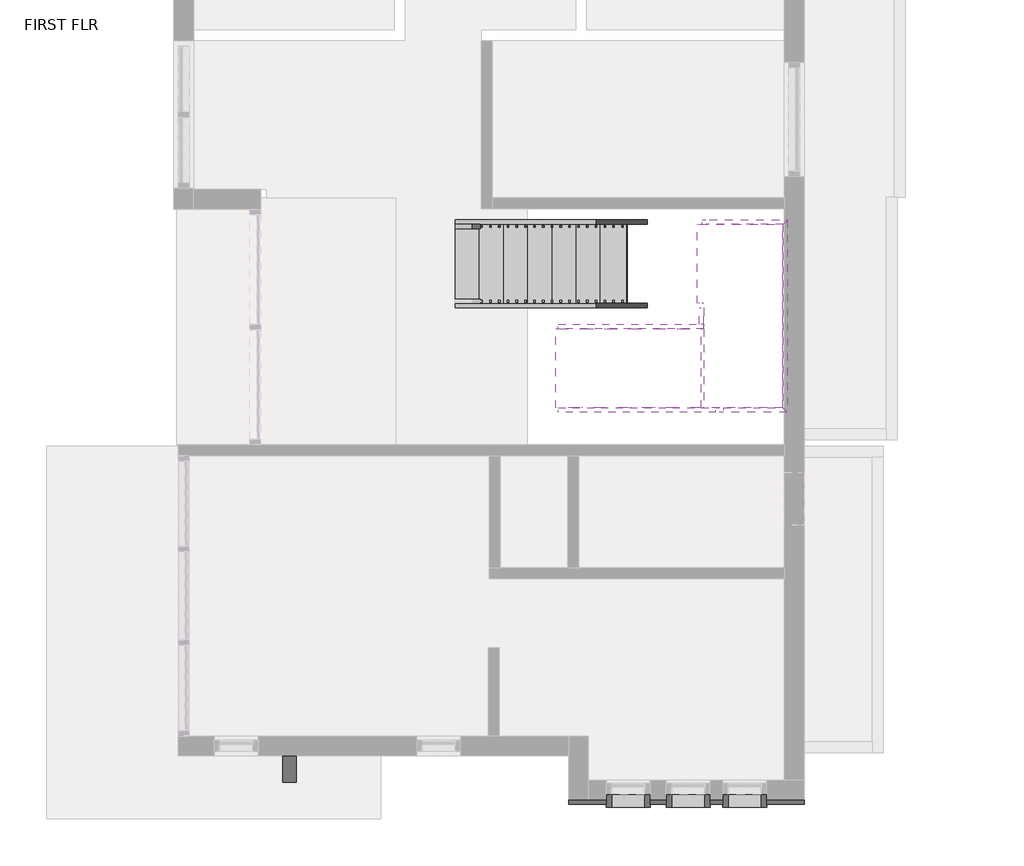
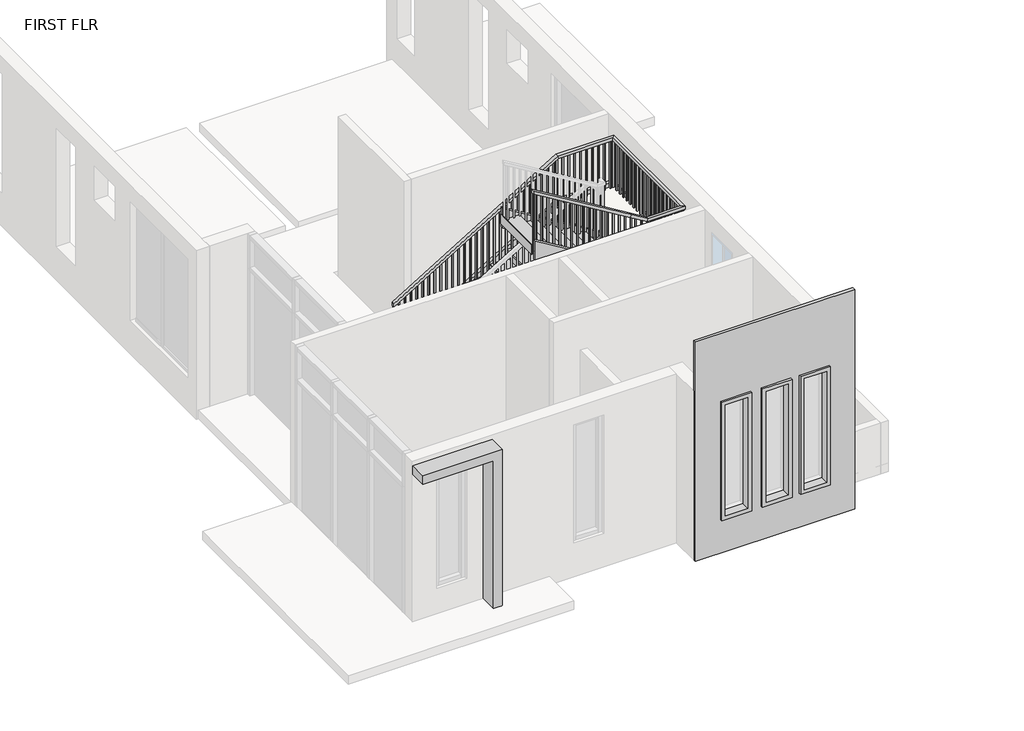
# One storey, part 4 of 4: 8 members, 3 proxies, 2 stair flights, 1 railing, 1 slab.
"""IFC4 building model written with IfcOpenShell, lengths in millimetres."""

from ifc_helpers import new_model, si_unit, frame, origin, place, context, project, spatial, polyline, outline, extrude, faceted_brep, transform, mapped, element, save
from components import generic_models_2_generic_models_2_65ba8ebd, generic_models_3_generic_models_3_7aa97fcf, generic_models_5_generic_models_5_32b8a8a5, non_monolithic_landing_a5fdca2b, stair_flight_bde5577f, stair_flight_bf40378d

model = new_model("IFC4")

# Units and contexts
model_context = context("Model", 3, world=origin())
ifc_project = project(units=[si_unit("LENGTHUNIT", "METRE", prefix="MILLI")], contexts=[model_context])

# Site, building, storey
site = spatial("IfcSite", under=ifc_project)
building = spatial("IfcBuilding", under=site)
storey = spatial("IfcBuildingStorey", under=building, Name="FIRST FLR", Elevation=3048.0)

# Proxies
placement = place(None, origin())
generic_models_2_generic_models_2_shape = generic_models_2_generic_models_2_65ba8ebd(model_context)
element("IfcBuildingElementProxy", 1, Name="Generic Models 2 : Generic Models 2", ObjectType="Generic Models 2 : Generic Models 2", at=placement, inside=storey, context=model_context, shape_type="MappedRepresentation", body=[
    mapped(generic_models_2_generic_models_2_shape, transform((0.0, 0.0, 0.0), x_axis=(1.0, 0.0, 0.0), y_axis=(0.0, 1.0, 0.0), z_axis=(0.0, 0.0, 1.0))),
])
generic_models_3_generic_models_3_shape = generic_models_3_generic_models_3_7aa97fcf(model_context)
element("IfcBuildingElementProxy", 2, Name="Generic Models 3 : Generic Models 3", ObjectType="Generic Models 3 : Generic Models 3", at=placement, inside=storey, context=model_context, shape_type="MappedRepresentation", body=[
    mapped(generic_models_3_generic_models_3_shape, transform((0.0, 0.0, 0.0), x_axis=(1.0, 0.0, 0.0), y_axis=(0.0, 1.0, 0.0), z_axis=(0.0, 0.0, 1.0))),
])
generic_models_5_generic_models_5_shape = generic_models_5_generic_models_5_32b8a8a5(model_context)
element("IfcBuildingElementProxy", 3, Name="Generic Models 5 : Generic Models 5", ObjectType="Generic Models 5 : Generic Models 5", at=placement, inside=storey, context=model_context, shape_type="MappedRepresentation", body=[
    mapped(generic_models_5_generic_models_5_shape, transform((0.0, 0.0, 0.0), x_axis=(1.0, 0.0, 0.0), y_axis=(0.0, 1.0, 0.0), z_axis=(0.0, 0.0, 1.0))),
])

# Members
element("IfcMember", 4, ObjectType="Stringer - 2\" Width", at=placement, inside=storey, context=model_context, shape_type="SweptSolid", body=[
    extrude(outline(polyline([(3260.114512, -9709.3703437), (3048.0, -9709.3703437), (3048.0, -9471.284832), (4682.0666667, -6775.074832), (4986.8666667, -6860.2292885), (3260.114512, -9709.3703437)])), frame((0.0, -5433.3504041, 0.0), z_axis=(0.0, 1.0, 0.0), x_axis=(0.0, 0.0, 1.0)), (0.0, 0.0, 1.0), 50.8),
])
element("IfcMember", 5, ObjectType="Stringer - 2\" Width", at=placement, inside=storey, context=model_context, shape_type="SweptSolid", body=[
    extrude(outline(polyline([(3260.114512, -9709.3703437), (3048.0, -9709.3703437), (3048.0, -9471.284832), (4641.9144067, -6841.3260609), (4986.8666667, -6841.3260609), (4986.8666667, -6860.2292885), (3260.114512, -9709.3703437)])), frame((0.0, -6398.5504041, 0.0), z_axis=(0.0, 1.0, 0.0), x_axis=(0.0, 0.0, 1.0)), (0.0, 0.0, 1.0), 50.8),
])
element("IfcMember", 6, ObjectType="Stringer - 2\" Width", at=placement, inside=storey, context=model_context, shape_type="SweptSolid", body=[
    extrude(outline(polyline([(4682.0666667, -6702.2215727), (4986.8666667, -6617.0671162), (6138.7811786, -8517.7260609), (5782.3724171, -8517.7260609), (4682.0666667, -6702.2215727)])), frame((0.0, -7604.2810793, 0.0), z_axis=(0.0, 1.0, 0.0), x_axis=(0.0, 0.0, 1.0)), (0.0, 0.0, 1.0), 50.8),
])
element("IfcMember", 7, ObjectType="Stringer - 2\" Width", at=placement, inside=storey, context=model_context, shape_type="SweptSolid", body=[
    extrude(outline(polyline([(4766.3724171, -6841.3260609), (5122.7811786, -6841.3260609), (6138.7811786, -8517.7260609), (5782.3724171, -8517.7260609), (4766.3724171, -6841.3260609)])), frame((0.0, -6639.0810793, 0.0), z_axis=(0.0, 1.0, 0.0), x_axis=(0.0, 0.0, 1.0)), (0.0, 0.0, 1.0), 50.8),
])
element("IfcMember", 8, ObjectType="Stringer - 2\" Width", at=placement, inside=storey, context=model_context, shape_type="Brep", body=[
    faceted_brep([(-6617.0671162, -7553.4810793, 4986.8666667), (-6617.0671162, -7604.2810793, 4986.8666667), (-5876.1260609, -7604.2810793, 4986.8666667), (-5926.9260609, -7553.4810793, 4986.8666667), (-6702.2215727, -7553.4810793, 4682.0666667), (-5926.9260609, -7553.4810793, 4682.0666667), (-6702.2215727, -7604.2810793, 4682.0666667), (-5876.1260609, -7604.2810793, 4682.0666667)], [[[0, 1, 2, 3]], [[4, 0, 3, 5]], [[6, 4, 5, 7]], [[1, 6, 7, 2]], [[1, 0, 4, 6]], [[2, 7, 5, 3]]]),
])
element("IfcMember", 9, ObjectType="Stringer - 2\" Width", at=placement, inside=storey, context=model_context, shape_type="SweptSolid", body=[
    extrude(outline(polyline([(-5876.1260609, -7604.2810793), (-5926.9260609, -7553.4810793), (-5926.9260609, -5433.3504041), (-5876.1260609, -5382.5504041), (-5876.1260609, -7604.2810793)])), frame((0.0, 0.0, 4682.0666667), z_axis=(0.0, 0.0, 1.0), x_axis=(1.0, 0.0, 0.0)), (0.0, 0.0, 1.0), 304.8),
])
element("IfcMember", 10, ObjectType="Stringer - 2\" Width", at=placement, inside=storey, context=model_context, shape_type="Brep", body=[
    faceted_brep([(-5926.9260609, -5433.3504041, 4986.8666667), (-5876.1260609, -5382.5504041, 4986.8666667), (-6860.2292885, -5382.5504041, 4986.8666667), (-6860.2292885, -5433.3504041, 4986.8666667), (-5926.9260609, -5433.3504041, 4682.0666667), (-6775.074832, -5433.3504041, 4682.0666667), (-5876.1260609, -5382.5504041, 4682.0666667), (-6775.074832, -5382.5504041, 4682.0666667)], [[[0, 1, 2, 3]], [[4, 0, 3, 5]], [[6, 4, 5, 7]], [[1, 6, 7, 2]], [[1, 0, 4, 6]], [[2, 7, 5, 3]]]),
])
element("IfcMember", 11, ObjectType="Stringer - 2\" Width", at=placement, inside=storey, context=model_context, shape_type="SweptSolid", body=[
    extrude(outline(polyline([(-6892.1260609, -6398.5504041), (-6841.3260609, -6398.5504041), (-6841.3260609, -6588.2810793), (-6892.1260609, -6588.2810793), (-6892.1260609, -6398.5504041)])), frame((0.0, 0.0, 4682.0666667), z_axis=(0.0, 0.0, 1.0), x_axis=(1.0, 0.0, 0.0)), (0.0, 0.0, 1.0), 304.8),
])

# Railing
element("IfcRailing", 12, ObjectType="Handrail - Rectangular", at=placement, inside=storey, context=model_context, shape_type="SolidModel", body=[
    faceted_brep([(-9709.3703437, -5433.3504041, 4131.7333333), (-9709.3703437, -5433.3504041, 4072.3318731), (-9709.3703437, -5484.1504041, 4072.3318731), (-9709.3703437, -5484.1504041, 4131.7333333), (-6915.3703437, -5433.3504041, 5825.0666667), (-6901.1779343, -5433.3504041, 5774.2666667), (-6901.1779343, -5484.1504041, 5774.2666667), (-6915.3703437, -5484.1504041, 5825.0666667), (-5926.9260609, -5433.3504041, 5825.0666667), (-5926.9260609, -5433.3504041, 5774.2666667), (-5977.7260609, -5484.1504041, 5774.2666667), (-5977.7260609, -5484.1504041, 5825.0666667), (-5926.9260609, -7553.4810793, 5825.0666667), (-5926.9260609, -7553.4810793, 5774.2666667), (-5977.7260609, -7502.6810793, 5774.2666667), (-5977.7260609, -7502.6810793, 5825.0666667), (-6561.9260609, -7553.4810793, 5825.0666667), (-6576.1184703, -7553.4810793, 5774.2666667), (-6576.1184703, -7502.6810793, 5774.2666667), (-6561.9260609, -7502.6810793, 5825.0666667), (-6841.3260609, -7553.4810793, 5994.4), (-6867.6557881, -7553.4810793, 5950.9559502), (-6867.6557881, -7502.6810793, 5950.9559502), (-6841.3260609, -7502.6810793, 5994.4), (-8517.7260609, -7553.4810793, 7010.4), (-8517.7260609, -7502.6810793, 7010.4), (-8517.7260609, -7502.6810793, 6950.9985397), (-8517.7260609, -7553.4810793, 6950.9985397)], [[[0, 1, 2, 3]], [[1, 0, 4, 5]], [[2, 1, 5, 6]], [[3, 2, 6, 7]], [[0, 3, 7, 4]], [[5, 4, 8, 9]], [[6, 5, 9, 10]], [[7, 6, 10, 11]], [[4, 7, 11, 8]], [[9, 8, 12, 13]], [[10, 9, 13, 14]], [[11, 10, 14, 15]], [[8, 11, 15, 12]], [[13, 12, 16, 17]], [[14, 13, 17, 18]], [[15, 14, 18, 19]], [[12, 15, 19, 16]], [[17, 16, 20, 21]], [[18, 17, 21, 22]], [[19, 18, 22, 23]], [[16, 19, 23, 20]], [[24, 25, 26, 27]], [[21, 20, 24, 27]], [[22, 21, 27, 26]], [[23, 22, 26, 25]], [[20, 23, 25, 24]]]),
    extrude(outline(polyline([(6925.9833882, -8476.4510609), (5926.6666667, -8476.4510609), (5926.6666667, -8457.4010609), (6914.4379337, -8457.4010609), (6925.9833882, -8476.4510609)])), frame((0.0, -7537.6060793, 0.0), z_axis=(0.0, 1.0, 0.0), x_axis=(0.0, 0.0, 1.0)), (0.0, 0.0, 1.0), 19.05),
    extrude(outline(polyline([(6864.4076307, -8374.8510609), (5926.6666667, -8374.8510609), (5926.6666667, -8355.8010609), (6852.8621761, -8355.8010609), (6864.4076307, -8374.8510609)])), frame((0.0, -7537.6060793, 0.0), z_axis=(0.0, 1.0, 0.0), x_axis=(0.0, 0.0, 1.0)), (0.0, 0.0, 1.0), 19.05),
    extrude(outline(polyline([(6802.8318731, -8273.2510609), (5926.6666667, -8273.2510609), (5926.6666667, -8254.2010609), (6791.2864185, -8254.2010609), (6802.8318731, -8273.2510609)])), frame((0.0, -7537.6060793, 0.0), z_axis=(0.0, 1.0, 0.0), x_axis=(0.0, 0.0, 1.0)), (0.0, 0.0, 1.0), 19.05),
    extrude(outline(polyline([(6741.2561155, -8171.6510609), (5757.3333333, -8171.6510609), (5757.3333333, -8152.6010609), (6729.710661, -8152.6010609), (6741.2561155, -8171.6510609)])), frame((0.0, -7537.6060793, 0.0), z_axis=(0.0, 1.0, 0.0), x_axis=(0.0, 0.0, 1.0)), (0.0, 0.0, 1.0), 19.05),
    extrude(outline(polyline([(6679.6803579, -8070.0510609), (5757.3333333, -8070.0510609), (5757.3333333, -8051.0010609), (6668.1349034, -8051.0010609), (6679.6803579, -8070.0510609)])), frame((0.0, -7537.6060793, 0.0), z_axis=(0.0, 1.0, 0.0), x_axis=(0.0, 0.0, 1.0)), (0.0, 0.0, 1.0), 19.05),
    extrude(outline(polyline([(6618.1046004, -7968.4510609), (5757.3333333, -7968.4510609), (5757.3333333, -7949.4010609), (6606.5591458, -7949.4010609), (6618.1046004, -7968.4510609)])), frame((0.0, -7537.6060793, 0.0), z_axis=(0.0, 1.0, 0.0), x_axis=(0.0, 0.0, 1.0)), (0.0, 0.0, 1.0), 19.05),
    extrude(outline(polyline([(6556.5288428, -7866.8510609), (5588.0, -7866.8510609), (5588.0, -7847.8010609), (6544.9833882, -7847.8010609), (6556.5288428, -7866.8510609)])), frame((0.0, -7537.6060793, 0.0), z_axis=(0.0, 1.0, 0.0), x_axis=(0.0, 0.0, 1.0)), (0.0, 0.0, 1.0), 19.05),
    extrude(outline(polyline([(6494.9530852, -7765.2510609), (5588.0, -7765.2510609), (5588.0, -7746.2010609), (6483.4076307, -7746.2010609), (6494.9530852, -7765.2510609)])), frame((0.0, -7537.6060793, 0.0), z_axis=(0.0, 1.0, 0.0), x_axis=(0.0, 0.0, 1.0)), (0.0, 0.0, 1.0), 19.05),
    extrude(outline(polyline([(6433.3773276, -7663.6510609), (5418.6666667, -7663.6510609), (5418.6666667, -7644.6010609), (6421.8318731, -7644.6010609), (6433.3773276, -7663.6510609)])), frame((0.0, -7537.6060793, 0.0), z_axis=(0.0, 1.0, 0.0), x_axis=(0.0, 0.0, 1.0)), (0.0, 0.0, 1.0), 19.05),
    extrude(outline(polyline([(6371.80157, -7562.0510609), (5418.6666667, -7562.0510609), (5418.6666667, -7543.0010609), (6360.2561155, -7543.0010609), (6371.80157, -7562.0510609)])), frame((0.0, -7537.6060793, 0.0), z_axis=(0.0, 1.0, 0.0), x_axis=(0.0, 0.0, 1.0)), (0.0, 0.0, 1.0), 19.05),
    extrude(outline(polyline([(6310.2258125, -7460.4510609), (5418.6666667, -7460.4510609), (5418.6666667, -7441.4010609), (6298.6803579, -7441.4010609), (6310.2258125, -7460.4510609)])), frame((0.0, -7537.6060793, 0.0), z_axis=(0.0, 1.0, 0.0), x_axis=(0.0, 0.0, 1.0)), (0.0, 0.0, 1.0), 19.05),
    extrude(outline(polyline([(6248.6500549, -7358.8510609), (5249.3333333, -7358.8510609), (5249.3333333, -7339.8010609), (6237.1046004, -7339.8010609), (6248.6500549, -7358.8510609)])), frame((0.0, -7537.6060793, 0.0), z_axis=(0.0, 1.0, 0.0), x_axis=(0.0, 0.0, 1.0)), (0.0, 0.0, 1.0), 19.05),
    extrude(outline(polyline([(6187.0742973, -7257.2510609), (5249.3333333, -7257.2510609), (5249.3333333, -7238.2010609), (6175.5288428, -7238.2010609), (6187.0742973, -7257.2510609)])), frame((0.0, -7537.6060793, 0.0), z_axis=(0.0, 1.0, 0.0), x_axis=(0.0, 0.0, 1.0)), (0.0, 0.0, 1.0), 19.05),
    extrude(outline(polyline([(6125.4985397, -7155.6510609), (5249.3333333, -7155.6510609), (5249.3333333, -7136.6010609), (6113.9530852, -7136.6010609), (6125.4985397, -7155.6510609)])), frame((0.0, -7537.6060793, 0.0), z_axis=(0.0, 1.0, 0.0), x_axis=(0.0, 0.0, 1.0)), (0.0, 0.0, 1.0), 19.05),
    extrude(outline(polyline([(6063.9227822, -7054.0510609), (5080.0, -7054.0510609), (5080.0, -7035.0010609), (6052.3773276, -7035.0010609), (6063.9227822, -7054.0510609)])), frame((0.0, -7537.6060793, 0.0), z_axis=(0.0, 1.0, 0.0), x_axis=(0.0, 0.0, 1.0)), (0.0, 0.0, 1.0), 19.05),
    extrude(outline(polyline([(6002.3470246, -6952.4510609), (5080.0, -6952.4510609), (5080.0, -6933.4010609), (5990.80157, -6933.4010609), (6002.3470246, -6952.4510609)])), frame((0.0, -7537.6060793, 0.0), z_axis=(0.0, 1.0, 0.0), x_axis=(0.0, 0.0, 1.0)), (0.0, 0.0, 1.0), 19.05),
    extrude(outline(polyline([(5894.5894488, -6774.6510609), (4910.6666667, -6774.6510609), (4910.6666667, -6755.6010609), (5883.0439943, -6755.6010609), (5894.5894488, -6774.6510609)])), frame((0.0, -7537.6060793, 0.0), z_axis=(0.0, 1.0, 0.0), x_axis=(0.0, 0.0, 1.0)), (0.0, 0.0, 1.0), 19.05),
    extrude(outline(polyline([(5833.0136913, -6673.0510609), (4910.6666667, -6673.0510609), (4910.6666667, -6654.0010609), (5821.4682367, -6654.0010609), (5833.0136913, -6673.0510609)])), frame((0.0, -7537.6060793, 0.0), z_axis=(0.0, 1.0, 0.0), x_axis=(0.0, 0.0, 1.0)), (0.0, 0.0, 1.0), 19.05),
    extrude(outline(polyline([(-6552.4010609, -7537.6060793), (-6571.4510609, -7537.6060793), (-6571.4510609, -7518.5560793), (-6552.4010609, -7518.5560793), (-6552.4010609, -7537.6060793)])), frame((0.0, 0.0, 4910.6666667), z_axis=(0.0, 0.0, 1.0), x_axis=(1.0, 0.0, 0.0)), (0.0, 0.0, 1.0), 863.6),
    extrude(outline(polyline([(-6450.8010609, -7537.6060793), (-6469.8510609, -7537.6060793), (-6469.8510609, -7518.5560793), (-6450.8010609, -7518.5560793), (-6450.8010609, -7537.6060793)])), frame((0.0, 0.0, 4910.6666667), z_axis=(0.0, 0.0, 1.0), x_axis=(1.0, 0.0, 0.0)), (0.0, 0.0, 1.0), 863.6),
    extrude(outline(polyline([(-6349.2010609, -7537.6060793), (-6368.2510609, -7537.6060793), (-6368.2510609, -7518.5560793), (-6349.2010609, -7518.5560793), (-6349.2010609, -7537.6060793)])), frame((0.0, 0.0, 4910.6666667), z_axis=(0.0, 0.0, 1.0), x_axis=(1.0, 0.0, 0.0)), (0.0, 0.0, 1.0), 863.6),
    extrude(outline(polyline([(-6247.6010609, -7537.6060793), (-6266.6510609, -7537.6060793), (-6266.6510609, -7518.5560793), (-6247.6010609, -7518.5560793), (-6247.6010609, -7537.6060793)])), frame((0.0, 0.0, 4910.6666667), z_axis=(0.0, 0.0, 1.0), x_axis=(1.0, 0.0, 0.0)), (0.0, 0.0, 1.0), 863.6),
    extrude(outline(polyline([(-6146.0010609, -7537.6060793), (-6165.0510609, -7537.6060793), (-6165.0510609, -7518.5560793), (-6146.0010609, -7518.5560793), (-6146.0010609, -7537.6060793)])), frame((0.0, 0.0, 4910.6666667), z_axis=(0.0, 0.0, 1.0), x_axis=(1.0, 0.0, 0.0)), (0.0, 0.0, 1.0), 863.6),
    extrude(outline(polyline([(-6044.4010609, -7537.6060793), (-6063.4510609, -7537.6060793), (-6063.4510609, -7518.5560793), (-6044.4010609, -7518.5560793), (-6044.4010609, -7537.6060793)])), frame((0.0, 0.0, 4910.6666667), z_axis=(0.0, 0.0, 1.0), x_axis=(1.0, 0.0, 0.0)), (0.0, 0.0, 1.0), 863.6),
    extrude(outline(polyline([(-5942.8010609, -7481.2254041), (-5942.8010609, -7500.2754041), (-5961.8510609, -7500.2754041), (-5961.8510609, -7481.2254041), (-5942.8010609, -7481.2254041)])), frame((0.0, 0.0, 4910.6666667), z_axis=(0.0, 0.0, 1.0), x_axis=(1.0, 0.0, 0.0)), (0.0, 0.0, 1.0), 863.6),
    extrude(outline(polyline([(-5942.8010609, -7379.6254041), (-5942.8010609, -7398.6754041), (-5961.8510609, -7398.6754041), (-5961.8510609, -7379.6254041), (-5942.8010609, -7379.6254041)])), frame((0.0, 0.0, 4910.6666667), z_axis=(0.0, 0.0, 1.0), x_axis=(1.0, 0.0, 0.0)), (0.0, 0.0, 1.0), 863.6),
    extrude(outline(polyline([(-5942.8010609, -7278.0254041), (-5942.8010609, -7297.0754041), (-5961.8510609, -7297.0754041), (-5961.8510609, -7278.0254041), (-5942.8010609, -7278.0254041)])), frame((0.0, 0.0, 4910.6666667), z_axis=(0.0, 0.0, 1.0), x_axis=(1.0, 0.0, 0.0)), (0.0, 0.0, 1.0), 863.6),
    extrude(outline(polyline([(-5942.8010609, -7176.4254041), (-5942.8010609, -7195.4754041), (-5961.8510609, -7195.4754041), (-5961.8510609, -7176.4254041), (-5942.8010609, -7176.4254041)])), frame((0.0, 0.0, 4910.6666667), z_axis=(0.0, 0.0, 1.0), x_axis=(1.0, 0.0, 0.0)), (0.0, 0.0, 1.0), 863.6),
    extrude(outline(polyline([(-5942.8010609, -7074.8254041), (-5942.8010609, -7093.8754041), (-5961.8510609, -7093.8754041), (-5961.8510609, -7074.8254041), (-5942.8010609, -7074.8254041)])), frame((0.0, 0.0, 4910.6666667), z_axis=(0.0, 0.0, 1.0), x_axis=(1.0, 0.0, 0.0)), (0.0, 0.0, 1.0), 863.6),
    extrude(outline(polyline([(-5942.8010609, -6973.2254041), (-5942.8010609, -6992.2754041), (-5961.8510609, -6992.2754041), (-5961.8510609, -6973.2254041), (-5942.8010609, -6973.2254041)])), frame((0.0, 0.0, 4910.6666667), z_axis=(0.0, 0.0, 1.0), x_axis=(1.0, 0.0, 0.0)), (0.0, 0.0, 1.0), 863.6),
    extrude(outline(polyline([(-5942.8010609, -6871.6254041), (-5942.8010609, -6890.6754041), (-5961.8510609, -6890.6754041), (-5961.8510609, -6871.6254041), (-5942.8010609, -6871.6254041)])), frame((0.0, 0.0, 4910.6666667), z_axis=(0.0, 0.0, 1.0), x_axis=(1.0, 0.0, 0.0)), (0.0, 0.0, 1.0), 863.6),
    extrude(outline(polyline([(-5942.8010609, -6770.0254041), (-5942.8010609, -6789.0754041), (-5961.8510609, -6789.0754041), (-5961.8510609, -6770.0254041), (-5942.8010609, -6770.0254041)])), frame((0.0, 0.0, 4910.6666667), z_axis=(0.0, 0.0, 1.0), x_axis=(1.0, 0.0, 0.0)), (0.0, 0.0, 1.0), 863.6),
    extrude(outline(polyline([(-5942.8010609, -6668.4254041), (-5942.8010609, -6687.4754041), (-5961.8510609, -6687.4754041), (-5961.8510609, -6668.4254041), (-5942.8010609, -6668.4254041)])), frame((0.0, 0.0, 4910.6666667), z_axis=(0.0, 0.0, 1.0), x_axis=(1.0, 0.0, 0.0)), (0.0, 0.0, 1.0), 863.6),
    extrude(outline(polyline([(-5942.8010609, -6566.8254041), (-5942.8010609, -6585.8754041), (-5961.8510609, -6585.8754041), (-5961.8510609, -6566.8254041), (-5942.8010609, -6566.8254041)])), frame((0.0, 0.0, 4910.6666667), z_axis=(0.0, 0.0, 1.0), x_axis=(1.0, 0.0, 0.0)), (0.0, 0.0, 1.0), 863.6),
    extrude(outline(polyline([(-5942.8010609, -6465.2254041), (-5942.8010609, -6484.2754041), (-5961.8510609, -6484.2754041), (-5961.8510609, -6465.2254041), (-5942.8010609, -6465.2254041)])), frame((0.0, 0.0, 4910.6666667), z_axis=(0.0, 0.0, 1.0), x_axis=(1.0, 0.0, 0.0)), (0.0, 0.0, 1.0), 863.6),
    extrude(outline(polyline([(-5942.8010609, -6363.6254041), (-5942.8010609, -6382.6754041), (-5961.8510609, -6382.6754041), (-5961.8510609, -6363.6254041), (-5942.8010609, -6363.6254041)])), frame((0.0, 0.0, 4910.6666667), z_axis=(0.0, 0.0, 1.0), x_axis=(1.0, 0.0, 0.0)), (0.0, 0.0, 1.0), 863.6),
    extrude(outline(polyline([(-5942.8010609, -6262.0254041), (-5942.8010609, -6281.0754041), (-5961.8510609, -6281.0754041), (-5961.8510609, -6262.0254041), (-5942.8010609, -6262.0254041)])), frame((0.0, 0.0, 4910.6666667), z_axis=(0.0, 0.0, 1.0), x_axis=(1.0, 0.0, 0.0)), (0.0, 0.0, 1.0), 863.6),
    extrude(outline(polyline([(-5942.8010609, -6160.4254041), (-5942.8010609, -6179.4754041), (-5961.8510609, -6179.4754041), (-5961.8510609, -6160.4254041), (-5942.8010609, -6160.4254041)])), frame((0.0, 0.0, 4910.6666667), z_axis=(0.0, 0.0, 1.0), x_axis=(1.0, 0.0, 0.0)), (0.0, 0.0, 1.0), 863.6),
    extrude(outline(polyline([(-5942.8010609, -6058.8254041), (-5942.8010609, -6077.8754041), (-5961.8510609, -6077.8754041), (-5961.8510609, -6058.8254041), (-5942.8010609, -6058.8254041)])), frame((0.0, 0.0, 4910.6666667), z_axis=(0.0, 0.0, 1.0), x_axis=(1.0, 0.0, 0.0)), (0.0, 0.0, 1.0), 863.6),
    extrude(outline(polyline([(-5942.8010609, -5957.2254041), (-5942.8010609, -5976.2754041), (-5961.8510609, -5976.2754041), (-5961.8510609, -5957.2254041), (-5942.8010609, -5957.2254041)])), frame((0.0, 0.0, 4910.6666667), z_axis=(0.0, 0.0, 1.0), x_axis=(1.0, 0.0, 0.0)), (0.0, 0.0, 1.0), 863.6),
    extrude(outline(polyline([(-5942.8010609, -5855.6254041), (-5942.8010609, -5874.6754041), (-5961.8510609, -5874.6754041), (-5961.8510609, -5855.6254041), (-5942.8010609, -5855.6254041)])), frame((0.0, 0.0, 4910.6666667), z_axis=(0.0, 0.0, 1.0), x_axis=(1.0, 0.0, 0.0)), (0.0, 0.0, 1.0), 863.6),
    extrude(outline(polyline([(-5942.8010609, -5754.0254041), (-5942.8010609, -5773.0754041), (-5961.8510609, -5773.0754041), (-5961.8510609, -5754.0254041), (-5942.8010609, -5754.0254041)])), frame((0.0, 0.0, 4910.6666667), z_axis=(0.0, 0.0, 1.0), x_axis=(1.0, 0.0, 0.0)), (0.0, 0.0, 1.0), 863.6),
    extrude(outline(polyline([(-5942.8010609, -5652.4254041), (-5942.8010609, -5671.4754041), (-5961.8510609, -5671.4754041), (-5961.8510609, -5652.4254041), (-5942.8010609, -5652.4254041)])), frame((0.0, 0.0, 4910.6666667), z_axis=(0.0, 0.0, 1.0), x_axis=(1.0, 0.0, 0.0)), (0.0, 0.0, 1.0), 863.6),
    extrude(outline(polyline([(-5942.8010609, -5550.8254041), (-5942.8010609, -5569.8754041), (-5961.8510609, -5569.8754041), (-5961.8510609, -5550.8254041), (-5942.8010609, -5550.8254041)])), frame((0.0, 0.0, 4910.6666667), z_axis=(0.0, 0.0, 1.0), x_axis=(1.0, 0.0, 0.0)), (0.0, 0.0, 1.0), 863.6),
    extrude(outline(polyline([(-6010.4953437, -5449.2254041), (-5991.4453437, -5449.2254041), (-5991.4453437, -5468.2754041), (-6010.4953437, -5468.2754041), (-6010.4953437, -5449.2254041)])), frame((0.0, 0.0, 4910.6666667), z_axis=(0.0, 0.0, 1.0), x_axis=(1.0, 0.0, 0.0)), (0.0, 0.0, 1.0), 863.6),
    extrude(outline(polyline([(-6112.0953437, -5449.2254041), (-6093.0453437, -5449.2254041), (-6093.0453437, -5468.2754041), (-6112.0953437, -5468.2754041), (-6112.0953437, -5449.2254041)])), frame((0.0, 0.0, 4910.6666667), z_axis=(0.0, 0.0, 1.0), x_axis=(1.0, 0.0, 0.0)), (0.0, 0.0, 1.0), 863.6),
    extrude(outline(polyline([(-6213.6953437, -5449.2254041), (-6194.6453437, -5449.2254041), (-6194.6453437, -5468.2754041), (-6213.6953437, -5468.2754041), (-6213.6953437, -5449.2254041)])), frame((0.0, 0.0, 4910.6666667), z_axis=(0.0, 0.0, 1.0), x_axis=(1.0, 0.0, 0.0)), (0.0, 0.0, 1.0), 863.6),
    extrude(outline(polyline([(-6315.2953437, -5449.2254041), (-6296.2453437, -5449.2254041), (-6296.2453437, -5468.2754041), (-6315.2953437, -5468.2754041), (-6315.2953437, -5449.2254041)])), frame((0.0, 0.0, 4910.6666667), z_axis=(0.0, 0.0, 1.0), x_axis=(1.0, 0.0, 0.0)), (0.0, 0.0, 1.0), 863.6),
    extrude(outline(polyline([(-6416.8953437, -5449.2254041), (-6397.8453437, -5449.2254041), (-6397.8453437, -5468.2754041), (-6416.8953437, -5468.2754041), (-6416.8953437, -5449.2254041)])), frame((0.0, 0.0, 4910.6666667), z_axis=(0.0, 0.0, 1.0), x_axis=(1.0, 0.0, 0.0)), (0.0, 0.0, 1.0), 863.6),
    extrude(outline(polyline([(-6518.4953437, -5449.2254041), (-6499.4453437, -5449.2254041), (-6499.4453437, -5468.2754041), (-6518.4953437, -5468.2754041), (-6518.4953437, -5449.2254041)])), frame((0.0, 0.0, 4910.6666667), z_axis=(0.0, 0.0, 1.0), x_axis=(1.0, 0.0, 0.0)), (0.0, 0.0, 1.0), 863.6),
    extrude(outline(polyline([(-6620.0953437, -5449.2254041), (-6601.0453437, -5449.2254041), (-6601.0453437, -5468.2754041), (-6620.0953437, -5468.2754041), (-6620.0953437, -5449.2254041)])), frame((0.0, 0.0, 4910.6666667), z_axis=(0.0, 0.0, 1.0), x_axis=(1.0, 0.0, 0.0)), (0.0, 0.0, 1.0), 863.6),
    extrude(outline(polyline([(-6721.6953437, -5449.2254041), (-6702.6453437, -5449.2254041), (-6702.6453437, -5468.2754041), (-6721.6953437, -5468.2754041), (-6721.6953437, -5449.2254041)])), frame((0.0, 0.0, 4910.6666667), z_axis=(0.0, 0.0, 1.0), x_axis=(1.0, 0.0, 0.0)), (0.0, 0.0, 1.0), 863.6),
    extrude(outline(polyline([(-6823.2953437, -5449.2254041), (-6804.2453437, -5449.2254041), (-6804.2453437, -5468.2754041), (-6823.2953437, -5468.2754041), (-6823.2953437, -5449.2254041)])), frame((0.0, 0.0, 4910.6666667), z_axis=(0.0, 0.0, 1.0), x_axis=(1.0, 0.0, 0.0)), (0.0, 0.0, 1.0), 863.6),
    extrude(outline(polyline([(5729.1046004, -6975.6953437), (4741.3333333, -6975.6953437), (4741.3333333, -6956.6453437), (5740.6500549, -6956.6453437), (5729.1046004, -6975.6953437)])), frame((0.0, -5468.2754041, 0.0), z_axis=(0.0, 1.0, 0.0), x_axis=(0.0, 0.0, 1.0)), (0.0, 0.0, 1.0), 19.05),
    extrude(outline(polyline([(5667.5288428, -7077.2953437), (4741.3333333, -7077.2953437), (4741.3333333, -7058.2453437), (5679.0742973, -7058.2453437), (5667.5288428, -7077.2953437)])), frame((0.0, -5468.2754041, 0.0), z_axis=(0.0, 1.0, 0.0), x_axis=(0.0, 0.0, 1.0)), (0.0, 0.0, 1.0), 19.05),
    extrude(outline(polyline([(5605.9530852, -7178.8953437), (4741.3333333, -7178.8953437), (4741.3333333, -7159.8453437), (5617.4985397, -7159.8453437), (5605.9530852, -7178.8953437)])), frame((0.0, -5468.2754041, 0.0), z_axis=(0.0, 1.0, 0.0), x_axis=(0.0, 0.0, 1.0)), (0.0, 0.0, 1.0), 19.05),
    extrude(outline(polyline([(5544.3773276, -7280.4953437), (4572.0, -7280.4953437), (4572.0, -7261.4453437), (5555.9227822, -7261.4453437), (5544.3773276, -7280.4953437)])), frame((0.0, -5468.2754041, 0.0), z_axis=(0.0, 1.0, 0.0), x_axis=(0.0, 0.0, 1.0)), (0.0, 0.0, 1.0), 19.05),
    extrude(outline(polyline([(5482.80157, -7382.0953437), (4572.0, -7382.0953437), (4572.0, -7363.0453437), (5494.3470246, -7363.0453437), (5482.80157, -7382.0953437)])), frame((0.0, -5468.2754041, 0.0), z_axis=(0.0, 1.0, 0.0), x_axis=(0.0, 0.0, 1.0)), (0.0, 0.0, 1.0), 19.05),
    extrude(outline(polyline([(5421.2258125, -7483.6953437), (4572.0, -7483.6953437), (4572.0, -7464.6453437), (5432.771267, -7464.6453437), (5421.2258125, -7483.6953437)])), frame((0.0, -5468.2754041, 0.0), z_axis=(0.0, 1.0, 0.0), x_axis=(0.0, 0.0, 1.0)), (0.0, 0.0, 1.0), 19.05),
    extrude(outline(polyline([(5359.6500549, -7585.2953437), (4402.6666667, -7585.2953437), (4402.6666667, -7566.2453437), (5371.1955094, -7566.2453437), (5359.6500549, -7585.2953437)])), frame((0.0, -5468.2754041, 0.0), z_axis=(0.0, 1.0, 0.0), x_axis=(0.0, 0.0, 1.0)), (0.0, 0.0, 1.0), 19.05),
    extrude(outline(polyline([(5298.0742973, -7686.8953437), (4402.6666667, -7686.8953437), (4402.6666667, -7667.8453437), (5309.6197519, -7667.8453437), (5298.0742973, -7686.8953437)])), frame((0.0, -5468.2754041, 0.0), z_axis=(0.0, 1.0, 0.0), x_axis=(0.0, 0.0, 1.0)), (0.0, 0.0, 1.0), 19.05),
    extrude(outline(polyline([(5236.4985397, -7788.4953437), (4233.3333333, -7788.4953437), (4233.3333333, -7769.4453437), (5248.0439943, -7769.4453437), (5236.4985397, -7788.4953437)])), frame((0.0, -5468.2754041, 0.0), z_axis=(0.0, 1.0, 0.0), x_axis=(0.0, 0.0, 1.0)), (0.0, 0.0, 1.0), 19.05),
    extrude(outline(polyline([(5174.9227822, -7890.0953437), (4233.3333333, -7890.0953437), (4233.3333333, -7871.0453437), (5186.4682367, -7871.0453437), (5174.9227822, -7890.0953437)])), frame((0.0, -5468.2754041, 0.0), z_axis=(0.0, 1.0, 0.0), x_axis=(0.0, 0.0, 1.0)), (0.0, 0.0, 1.0), 19.05),
    extrude(outline(polyline([(5113.3470246, -7991.6953437), (4233.3333333, -7991.6953437), (4233.3333333, -7972.6453437), (5124.8924791, -7972.6453437), (5113.3470246, -7991.6953437)])), frame((0.0, -5468.2754041, 0.0), z_axis=(0.0, 1.0, 0.0), x_axis=(0.0, 0.0, 1.0)), (0.0, 0.0, 1.0), 19.05),
    extrude(outline(polyline([(5051.771267, -8093.2953437), (4064.0, -8093.2953437), (4064.0, -8074.2453437), (5063.3167216, -8074.2453437), (5051.771267, -8093.2953437)])), frame((0.0, -5468.2754041, 0.0), z_axis=(0.0, 1.0, 0.0), x_axis=(0.0, 0.0, 1.0)), (0.0, 0.0, 1.0), 19.05),
    extrude(outline(polyline([(4990.1955094, -8194.8953437), (4064.0, -8194.8953437), (4064.0, -8175.8453437), (5001.740964, -8175.8453437), (4990.1955094, -8194.8953437)])), frame((0.0, -5468.2754041, 0.0), z_axis=(0.0, 1.0, 0.0), x_axis=(0.0, 0.0, 1.0)), (0.0, 0.0, 1.0), 19.05),
    extrude(outline(polyline([(4928.6197519, -8296.4953437), (4064.0, -8296.4953437), (4064.0, -8277.4453437), (4940.1652064, -8277.4453437), (4928.6197519, -8296.4953437)])), frame((0.0, -5468.2754041, 0.0), z_axis=(0.0, 1.0, 0.0), x_axis=(0.0, 0.0, 1.0)), (0.0, 0.0, 1.0), 19.05),
    extrude(outline(polyline([(4867.0439943, -8398.0953437), (3894.6666667, -8398.0953437), (3894.6666667, -8379.0453437), (4878.5894488, -8379.0453437), (4867.0439943, -8398.0953437)])), frame((0.0, -5468.2754041, 0.0), z_axis=(0.0, 1.0, 0.0), x_axis=(0.0, 0.0, 1.0)), (0.0, 0.0, 1.0), 19.05),
    extrude(outline(polyline([(4805.4682367, -8499.6953437), (3894.6666667, -8499.6953437), (3894.6666667, -8480.6453437), (4817.0136913, -8480.6453437), (4805.4682367, -8499.6953437)])), frame((0.0, -5468.2754041, 0.0), z_axis=(0.0, 1.0, 0.0), x_axis=(0.0, 0.0, 1.0)), (0.0, 0.0, 1.0), 19.05),
    extrude(outline(polyline([(4743.8924791, -8601.2953437), (3894.6666667, -8601.2953437), (3894.6666667, -8582.2453437), (4755.4379337, -8582.2453437), (4743.8924791, -8601.2953437)])), frame((0.0, -5468.2754041, 0.0), z_axis=(0.0, 1.0, 0.0), x_axis=(0.0, 0.0, 1.0)), (0.0, 0.0, 1.0), 19.05),
    extrude(outline(polyline([(4682.3167216, -8702.8953437), (3725.3333333, -8702.8953437), (3725.3333333, -8683.8453437), (4693.8621761, -8683.8453437), (4682.3167216, -8702.8953437)])), frame((0.0, -5468.2754041, 0.0), z_axis=(0.0, 1.0, 0.0), x_axis=(0.0, 0.0, 1.0)), (0.0, 0.0, 1.0), 19.05),
    extrude(outline(polyline([(4620.740964, -8804.4953437), (3725.3333333, -8804.4953437), (3725.3333333, -8785.4453437), (4632.2864185, -8785.4453437), (4620.740964, -8804.4953437)])), frame((0.0, -5468.2754041, 0.0), z_axis=(0.0, 1.0, 0.0), x_axis=(0.0, 0.0, 1.0)), (0.0, 0.0, 1.0), 19.05),
    extrude(outline(polyline([(4559.1652064, -8906.0953437), (3556.0, -8906.0953437), (3556.0, -8887.0453437), (4570.710661, -8887.0453437), (4559.1652064, -8906.0953437)])), frame((0.0, -5468.2754041, 0.0), z_axis=(0.0, 1.0, 0.0), x_axis=(0.0, 0.0, 1.0)), (0.0, 0.0, 1.0), 19.05),
    extrude(outline(polyline([(4497.5894488, -9007.6953437), (3556.0, -9007.6953437), (3556.0, -8988.6453437), (4509.1349034, -8988.6453437), (4497.5894488, -9007.6953437)])), frame((0.0, -5468.2754041, 0.0), z_axis=(0.0, 1.0, 0.0), x_axis=(0.0, 0.0, 1.0)), (0.0, 0.0, 1.0), 19.05),
    extrude(outline(polyline([(4436.0136913, -9109.2953437), (3556.0, -9109.2953437), (3556.0, -9090.2453437), (4447.5591458, -9090.2453437), (4436.0136913, -9109.2953437)])), frame((0.0, -5468.2754041, 0.0), z_axis=(0.0, 1.0, 0.0), x_axis=(0.0, 0.0, 1.0)), (0.0, 0.0, 1.0), 19.05),
    extrude(outline(polyline([(4374.4379337, -9210.8953437), (3386.6666667, -9210.8953437), (3386.6666667, -9191.8453437), (4385.9833882, -9191.8453437), (4374.4379337, -9210.8953437)])), frame((0.0, -5468.2754041, 0.0), z_axis=(0.0, 1.0, 0.0), x_axis=(0.0, 0.0, 1.0)), (0.0, 0.0, 1.0), 19.05),
    extrude(outline(polyline([(4312.8621761, -9312.4953437), (3386.6666667, -9312.4953437), (3386.6666667, -9293.4453437), (4324.4076307, -9293.4453437), (4312.8621761, -9312.4953437)])), frame((0.0, -5468.2754041, 0.0), z_axis=(0.0, 1.0, 0.0), x_axis=(0.0, 0.0, 1.0)), (0.0, 0.0, 1.0), 19.05),
    extrude(outline(polyline([(4251.2864185, -9414.0953437), (3386.6666667, -9414.0953437), (3386.6666667, -9395.0453437), (4262.8318731, -9395.0453437), (4251.2864185, -9414.0953437)])), frame((0.0, -5468.2754041, 0.0), z_axis=(0.0, 1.0, 0.0), x_axis=(0.0, 0.0, 1.0)), (0.0, 0.0, 1.0), 19.05),
    extrude(outline(polyline([(4189.710661, -9515.6953437), (3217.3333333, -9515.6953437), (3217.3333333, -9496.6453437), (4201.2561155, -9496.6453437), (4189.710661, -9515.6953437)])), frame((0.0, -5468.2754041, 0.0), z_axis=(0.0, 1.0, 0.0), x_axis=(0.0, 0.0, 1.0)), (0.0, 0.0, 1.0), 19.05),
    extrude(outline(polyline([(4128.1349034, -9617.2953437), (3217.3333333, -9617.2953437), (3217.3333333, -9598.2453437), (4139.6803579, -9598.2453437), (4128.1349034, -9617.2953437)])), frame((0.0, -5468.2754041, 0.0), z_axis=(0.0, 1.0, 0.0), x_axis=(0.0, 0.0, 1.0)), (0.0, 0.0, 1.0), 19.05),
    extrude(outline(polyline([(5940.771267, -6850.8510609), (4910.6666667, -6850.8510609), (4910.6666667, -6831.8010609), (5929.2258125, -6831.8010609), (5940.771267, -6850.8510609)])), frame((0.0, -7537.6060793, 0.0), z_axis=(0.0, 1.0, 0.0), x_axis=(0.0, 0.0, 1.0)), (0.0, 0.0, 1.0), 19.05),
    extrude(outline(polyline([(-5942.8010609, -7518.5560793), (-5942.8010609, -7537.6060793), (-5961.8510609, -7537.6060793), (-5961.8510609, -7518.5560793), (-5942.8010609, -7518.5560793)])), frame((0.0, 0.0, 4910.6666667), z_axis=(0.0, 0.0, 1.0), x_axis=(1.0, 0.0, 0.0)), (0.0, 0.0, 1.0), 863.6),
    extrude(outline(polyline([(-5961.8510609, -5449.2254041), (-5942.8010609, -5449.2254041), (-5942.8010609, -5468.2754041), (-5961.8510609, -5468.2754041), (-5961.8510609, -5449.2254041)])), frame((0.0, 0.0, 4910.6666667), z_axis=(0.0, 0.0, 1.0), x_axis=(1.0, 0.0, 0.0)), (0.0, 0.0, 1.0), 863.6),
    extrude(outline(polyline([(5759.8924791, -6924.8953437), (4910.6666667, -6924.8953437), (4910.6666667, -6905.8453437), (5771.4379337, -6905.8453437), (5759.8924791, -6924.8953437)])), frame((0.0, -5468.2754041, 0.0), z_axis=(0.0, 1.0, 0.0), x_axis=(0.0, 0.0, 1.0)), (0.0, 0.0, 1.0), 19.05),
    extrude(outline(polyline([(6950.9985397, -8517.7260609), (5926.6666667, -8517.7260609), (5926.6666667, -8498.6760609), (6939.4530852, -8498.6760609), (6950.9985397, -8517.7260609)])), frame((0.0, -7537.6060793, 0.0), z_axis=(0.0, 1.0, 0.0), x_axis=(0.0, 0.0, 1.0)), (0.0, 0.0, 1.0), 19.05),
    extrude(outline(polyline([(4072.3318731, -9709.3703437), (3217.3333333, -9709.3703437), (3217.3333333, -9690.3203437), (4083.8773276, -9690.3203437), (4072.3318731, -9709.3703437)])), frame((0.0, -5468.2754041, 0.0), z_axis=(0.0, 1.0, 0.0), x_axis=(0.0, 0.0, 1.0)), (0.0, 0.0, 1.0), 19.05),
])

# Slab
non_monolithic_landing_shape = non_monolithic_landing_a5fdca2b(model_context)
element("IfcSlab", 13, ObjectType="Non-Monolithic Landing", at=placement, inside=storey, context=model_context, shape_type="MappedRepresentation", body=[
    mapped(non_monolithic_landing_shape, transform((0.0, 0.0, 0.0), x_axis=(1.0, 0.0, 0.0), y_axis=(0.0, 1.0, 0.0), z_axis=(0.0, 0.0, 1.0))),
])

# Stair flights
stair_flight_shape = stair_flight_bde5577f(model_context)
element("IfcStairFlight", 14, ObjectType="2\" Tread 1\" Nosing 1/4\" Riser", at=placement, inside=storey, context=model_context, shape_type="MappedRepresentation", body=[
    mapped(stair_flight_shape, transform((0.0, 0.0, 0.0), x_axis=(1.0, 0.0, 0.0), y_axis=(0.0, 1.0, 0.0), z_axis=(0.0, 0.0, 1.0))),
])
stair_flight_2_shape = stair_flight_bf40378d(model_context)
element("IfcStairFlight", 15, ObjectType="2\" Tread 1\" Nosing 1/4\" Riser", at=placement, inside=storey, context=model_context, shape_type="MappedRepresentation", body=[
    mapped(stair_flight_2_shape, transform((0.0, 0.0, 0.0), x_axis=(1.0, 0.0, 0.0), y_axis=(0.0, 1.0, 0.0), z_axis=(0.0, 0.0, 1.0))),
])

save(model, "model.ifc")

# Revit data of these elements
# Type "Handrail - Rectangular"
#   Assembly Code = "C2010400"
#   built-in parameter 1008612 = 0.0416667 (stored number, unit not read)
#   built-in parameter 1008611 = 0.0416667 (stored number, unit not read)
#   built-in parameter 1008609 = 0.333333 (stored number, unit not read)
#   built-in parameter 1008604 = 0.166667 (stored number, unit not read)
#   built-in parameter 1008603 = 0.166667 (stored number, unit not read)
#   Railing Height = 3' - 0"
#   built-in parameter 1008630 = 2
#   built-in parameter 1008610 = 2
#   built-in parameter 1008618 = Baluster - Square : 3/4"
# Element 1 (IfcBuildingElementProxy, "Generic Models 2 : Generic Models 2")
#   Phase Created = New Construction
#   Materials on its faces: "GREY COLOUR FRAME"
# Element 2 (IfcBuildingElementProxy, "Generic Models 3 : Generic Models 3")
#   Phase Created = New Construction
#   Materials on its faces: "GREY COLOUR FRAME(1)"
# Element 3 (IfcBuildingElementProxy, "Generic Models 5 : Generic Models 5")
#   Phase Created = New Construction
#   Materials on its faces: "GREY COLOUR FRAME(1)"
# Elements 4, 5 (IfcMember, "Stringer - 2\" Width")
#   Phase Created = New Construction
#   Materials on its faces: "MARBLE FLOORING 1'"
# Elements 6, 7, 8, 9, 10, 11 (IfcMember, "Stringer - 2\" Width")
#   Phase Created = New Construction
# Element 12 (IfcRailing, "Handrail - Rectangular")
#   Phase Created = New Construction
# Element 13 (IfcSlab, "Non-Monolithic Landing")
#   Phase Created = New Construction
# Elements 14, 15 (IfcStairFlight, "2\" Tread 1\" Nosing 1/4\" Riser")
#   Phase Created = New Construction
# Materials
#   "GREY COLOUR FRAME": class "Generic", colour RGB 120 120 120, transparency 0, Cost = 0
#   "GREY COLOUR FRAME(1)": class "Generic", colour RGB 120 120 120, transparency 0, Cost = 0
#   "MARBLE FLOORING 1'": class "Generic", colour RGB 120 120 120, transparency 0, Cost = 0
